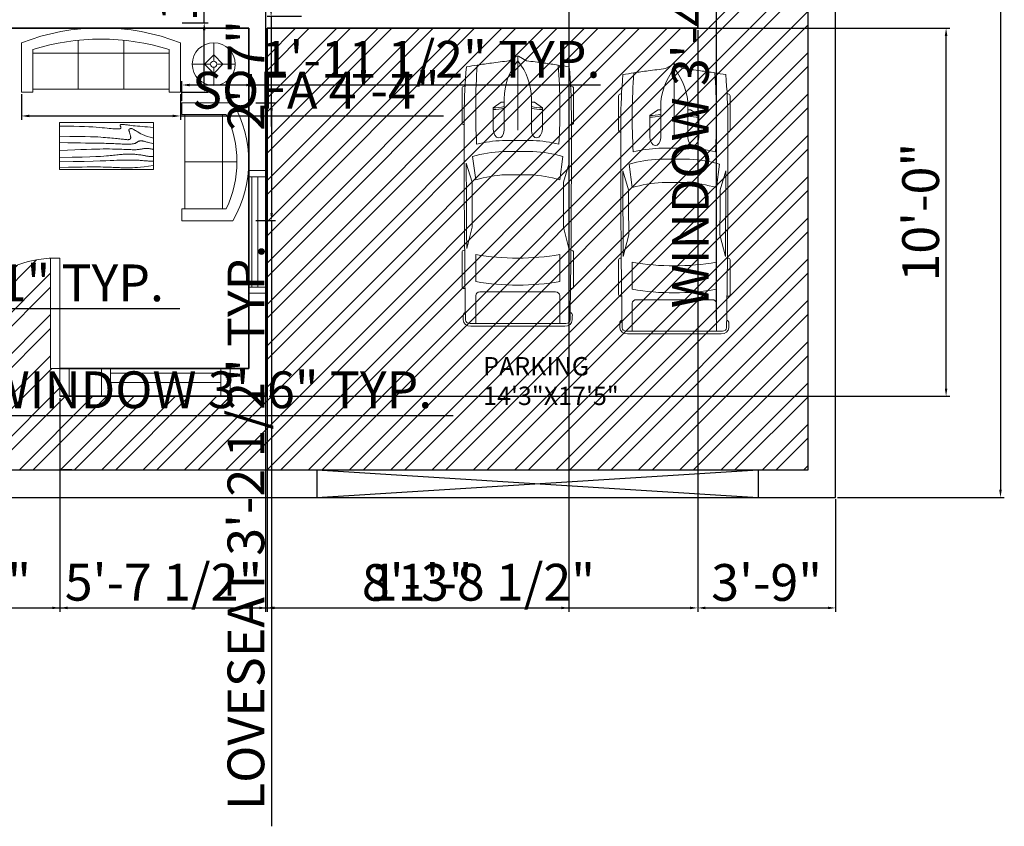
# Model space of a CAD drawing. Units: inches. Extents: x 2297 to 3143, y 440 to 1351.
# Tile 3 of 6: x 2725 to 3047, y 440 to 703. Entities that reach past the tile are written whole.
import ezdxf

# ---------------------------------------------------------------- set-up
doc = ezdxf.new("R2010")
doc.units = ezdxf.units.IN
for name, color, linetype, lineweight in [('A-ANNO-DIMS', 2, 'Continuous', 18), ('A-AREA-IDEN', 7, 'Continuous', 18), ('A-DOOR', 4, 'Continuous', 20), ('A-FURN', 8, 'Continuous', 18), ('A-GLAZ', 4, 'Continuous', 18), ('A-WALL', 7, 'Continuous', 35), ('C-PKNG-VEH', 8, 'Continuous', 13), ('C-PROP', 7, 'Continuous', 25), ('C-SITE-PATT', 252, 'Continuous', 13), ('E-LITE', 9, 'Continuous', 13)]:
    doc.layers.add(name, color=color, linetype=linetype, lineweight=lineweight)
doc.styles.get("Standard").update_dxf_attribs({"font": 'arial.ttf'})
doc.dimstyles.new('ISO-25', dxfattribs={"dimtxt": 12, "dimasz": 2.5, "dimexe": 1.25, "dimexo": 0.625, "dimtad": 1, "dimdec": 1, "dimlunit": 3, "dimtxsty": 'Standard', "dimcen": 2.5, "dimadec": 0, "dimazin": 0, "dimtfac": 1, "dimtdec": 1, "dimtmove": 0, "dimatfit": 3, "dimfxl": 1, "dimarcsym": 0})

# ---------------------------------------------------------------- blocks, each defined once
blk = doc.blocks.new('Sofa - Roundback Loveseat 5 ft.')
for p, q in [((0, -32.44198), (0, -5.99998)), ((-24, -33.99998), (-24, -11.46958)), ((-23.9998, -13.38178), (23.99986, -13.38178)), ((24.00004, -33.99998), (24.00004, -11.46958)), ((-24, -32.44198), (24.00004, -32.44198))]:
    blk.add_line(p, q)
for points in [[(-24, -33.99998), (-30, -33.99998), (-30, -7.99998)], [(30.00004, -7.99998), (30.00004, -33.99998), (24.00004, -33.99998)]]:
    blk.add_lwpolyline(points)
for centre, radius, start, end in [((0, -60.24998), 60.24998, 60.13715, 119.8628), ((0, -61.38438), 55.38444, 64.32083, 115.6792)]:
    blk.add_arc(centre, radius, start, end)
blk = doc.blocks.new('Table - Rectangular Woodgrain 60 x 30 in.')
for p, q in [((0, 0), (0, -30)), ((60, 0), (0, 0)), ((60, -30), (60, 0)), ((0, -30), (60, -30))]:
    blk.add_line(p, q)
for points in [[(0, -2.4), (4.8155, -2.418), (9.0302, -2.4688), (12.709, -2.5477), (15.9167, -2.65), (18.7181, -2.7711), (21.1781, -2.9063), (23.3616, -3.0508), (25.3333, -3.2), (27.1477, -3.3495), (28.8172, -3.4958), (30.3437, -3.636), (31.7291, -3.7667), (32.9756, -3.8849), (34.0849, -3.9875), (35.059, -4.0714), (35.9, -4.1334), (36.6114, -4.1711), (37.2041, -4.1854), (37.6906, -4.1779), (38.0833, -4.15), (38.3948, -4.1034), (38.6375, -4.0396), (38.8239, -3.9602), (38.9666, -3.8667), (39.0764, -3.7608), (39.1573, -3.6448), (39.2116, -3.521), (39.2416, -3.3917), (39.2498, -3.2593), (39.2385, -3.1261), (39.21, -2.9944), (39.1666, -2.8667), (39.111, -2.7447), (39.0468, -2.6281), (38.978, -2.5163), (38.9083, -2.4083), (38.8418, -2.3035), (38.7823, -2.201), (38.7337, -2.1001), (38.7, -2), (38.6844, -1.9003), (38.6875, -1.8021), (38.7094, -1.707), (38.75, -1.6167), (38.8094, -1.5326), (38.8875, -1.4563), (38.9844, -1.3893), (39.1, -1.3333), (39.2351, -1.2896), (39.3937, -1.2583), (39.5804, -1.2396), (39.8, -1.2333), (40.057, -1.2396), (40.3562, -1.2583), (40.7023, -1.2896), (41.1, -1.3333), (41.5547, -1.3895), (42.0755, -1.4573), (42.6721, -1.5361), (43.3542, -1.625), (44.1316, -1.7233), (45.014, -1.8302), (46.0114, -1.9449), (47.1333, -2.0667), (48.3862, -2.1947), (49.7625, -2.3281), (51.2513, -2.4663), (52.8416, -2.6083), (54.5226, -2.7535), (56.2833, -2.9011), (58.1127, -3.0501), (60, -3.2)], [(0, -9.2), (6.5759, -9.0858), (11.9385, -9.0365), (16.2527, -9.0418), (19.6833, -9.0917), (22.3952, -9.1759), (24.5531, -9.2844), (26.322, -9.4069), (27.8666, -9.5333), (29.3241, -9.6553), (30.7203, -9.7719), (32.0532, -9.8837), (33.3208, -9.9917), (34.5213, -10.0965), (35.6526, -10.199), (36.7128, -10.2999), (37.7, -10.4), (38.6129, -10.4996), (39.4531, -10.5969), (40.223, -10.6895), (40.925, -10.775), (41.5613, -10.8512), (42.1344, -10.9156), (42.6465, -10.966), (43.1, -11), (43.4976, -11.0158), (43.8437, -11.0136), (44.143, -10.9942), (44.4, -10.9583), (44.6195, -10.9069), (44.8062, -10.8406), (44.9648, -10.7603), (45.1, -10.6667), (45.2155, -10.5598), (45.3114, -10.4365), (45.3871, -10.2929), (45.4416, -10.125), (45.4743, -9.929), (45.4844, -9.7011), (45.4709, -9.4371), (45.4333, -9.1333), (45.3716, -8.7883), (45.2896, -8.4104), (45.1919, -8.0107), (45.0833, -7.6), (44.9685, -7.1893), (44.8521, -6.7896), (44.7388, -6.4117), (44.6333, -6.0667), (44.54, -5.7628), (44.4614, -5.4979), (44.4001, -5.2675), (44.3583, -5.0667), (44.3384, -4.8909), (44.3427, -4.7354), (44.3736, -4.5956), (44.4333, -4.4667), (44.5236, -4.3453), (44.6427, -4.2333), (44.7884, -4.1339), (44.9583, -4.05), (45.1501, -3.9849), (45.3614, -3.9417), (45.59, -3.9234), (45.8333, -3.9333), (46.0915, -3.9749), (46.3734, -4.0531), (46.6906, -4.1736), (47.0542, -4.3417), (47.4756, -4.5629), (47.9661, -4.8427), (48.5372, -5.1866), (49.2, -5.6), (49.9676, -6.0844), (50.8594, -6.625), (51.8965, -7.2031), (53.1, -7.8), (54.491, -8.3969), (56.0906, -8.975), (57.9199, -9.5156), (60, -10)], [(0, -12.8), (5.1847, -12.9322), (9.6213, -13.0323), (13.3963, -13.1059), (16.5958, -13.1583), (19.3063, -13.1952), (21.614, -13.2219), (23.6054, -13.2439), (25.3666, -13.2667), (26.9728, -13.2947), (28.4531, -13.3281), (29.8256, -13.3663), (31.1083, -13.4083), (32.3191, -13.4535), (33.476, -13.501), (34.597, -13.5501), (35.7, -13.6), (36.7984, -13.6497), (37.8875, -13.6979), (38.9578, -13.743), (40, -13.7833), (41.0047, -13.8174), (41.9625, -13.8438), (42.864, -13.8607), (43.7, -13.8667), (44.4631, -13.8604), (45.1552, -13.8417), (45.7801, -13.8104), (46.3416, -13.7667), (46.8439, -13.7104), (47.2906, -13.6417), (47.6858, -13.5604), (48.0333, -13.4667), (48.3375, -13.3608), (48.6042, -13.2448), (48.8396, -13.121), (49.05, -12.9917), (49.2417, -12.8593), (49.4208, -12.7261), (49.5937, -12.5944), (49.7667, -12.4667), (49.9452, -12.3451), (50.1323, -12.2313), (50.3303, -12.1268), (50.5416, -12.0333), (50.7686, -11.9524), (51.0135, -11.8854), (51.2788, -11.8341), (51.5666, -11.8), (51.8785, -11.7843), (52.2116, -11.7865), (52.562, -11.8059), (52.926, -11.8417), (53.2998, -11.8931), (53.6795, -11.9594), (54.0614, -12.0397), (54.4416, -12.1333), (54.8223, -12.2401), (55.2293, -12.3625), (55.6942, -12.5037), (56.2489, -12.6667), (56.9251, -12.8547), (57.7545, -13.0708), (58.7689, -13.3182), (60, -13.6)], [(0, -18), (5.124, -17.7273), (9.6609, -17.5057), (13.6705, -17.3303), (17.2125, -17.1958), (20.3467, -17.0973), (23.1328, -17.0297), (25.6307, -16.9878), (27.9, -16.9667), (29.9928, -16.9617), (31.9302, -16.9703), (33.7254, -16.9907), (35.3917, -17.0208), (36.9423, -17.0588), (38.3906, -17.1026), (39.7499, -17.1503), (41.0333, -17.2), (42.2519, -17.2496), (43.4073, -17.2969), (44.4986, -17.3395), (45.525, -17.375), (46.4858, -17.4012), (47.3802, -17.4156), (48.2074, -17.416), (48.9667, -17.4), (49.6583, -17.3662), (50.2872, -17.3167), (50.8595, -17.2547), (51.3812, -17.1833), (51.8584, -17.1057), (52.2971, -17.025), (52.7034, -16.9443), (53.0833, -16.8667), (53.443, -16.7951), (53.789, -16.7313), (54.128, -16.6768), (54.4666, -16.6334), (54.8115, -16.6024), (55.1693, -16.5854), (55.5465, -16.5841), (55.95, -16.6), (56.3828, -16.6337), (56.8346, -16.6823), (57.2915, -16.7418), (57.7396, -16.8084), (58.165, -16.878), (58.5539, -16.9469), (58.8924, -17.0111), (59.1666, -17.0667), (59.3679, -17.1107), (59.5078, -17.1438), (59.6032, -17.1675), (59.6708, -17.1833), (59.7275, -17.193), (59.7901, -17.1979), (59.8753, -17.1998), (60, -17.2)], [(0, -22.4), (8.0098, -22.2501), (14.4094, -22.1011), (19.4168, -21.9535), (23.25, -21.8083), (26.1269, -21.6663), (28.2656, -21.5281), (29.884, -21.3947), (31.2, -21.2667), (32.3967, -21.1448), (33.5172, -21.0292), (34.5697, -20.9198), (35.5625, -20.8167), (36.5037, -20.7198), (37.4015, -20.6292), (38.2642, -20.5448), (39.1, -20.4667), (39.9164, -20.3951), (40.7187, -20.3313), (41.5117, -20.2768), (42.3, -20.2333), (43.0883, -20.2024), (43.8812, -20.1854), (44.6836, -20.1841), (45.5, -20.2), (46.3328, -20.234), (47.1747, -20.2844), (48.0163, -20.3488), (48.8479, -20.425), (49.66, -20.5106), (50.4429, -20.6031), (51.1872, -20.7004), (51.8833, -20.8), (52.5246, -20.8999), (53.1166, -20.9995), (53.6681, -21.0983), (54.1875, -21.1958), (54.6834, -21.2919), (55.1646, -21.3859), (55.6394, -21.4777), (56.1167, -21.5667), (56.6028, -21.6515), (57.0961, -21.7266), (57.5929, -21.7852), (58.0896, -21.8208), (58.5823, -21.8268), (59.0674, -21.7964), (59.5412, -21.723), (60, -21.6)], [(0, -25.2), (8.6355, -25.0504), (15.7026, -24.9031), (21.4049, -24.7606), (25.9458, -24.625), (29.529, -24.4988), (32.3578, -24.3844), (34.6359, -24.284), (36.5667, -24.2), (38.3213, -24.1341), (39.9417, -24.0854), (41.437, -24.0523), (42.8167, -24.0333), (44.0901, -24.0268), (45.2667, -24.0313), (46.3557, -24.0451), (47.3667, -24.0667), (48.309, -24.0947), (49.1928, -24.1287), (50.0284, -24.168), (50.826, -24.2125), (51.5959, -24.2617), (52.3483, -24.3151), (53.0935, -24.3725), (53.8417, -24.4334), (54.6009, -24.497), (55.3699, -24.561), (56.1454, -24.6226), (56.9239, -24.6792), (57.7021, -24.7279), (58.4764, -24.7662), (59.2435, -24.7911), (60, -24.8)], [(0, -28.8), (5.6867, -28.6681), (10.45, -28.5698), (14.407, -28.5012), (17.675, -28.4584), (20.3711, -28.4374), (22.6125, -28.4344), (24.5164, -28.4455), (26.2, -28.4667), (27.762, -28.4947), (29.2276, -28.5281), (30.6033, -28.5663), (31.8958, -28.6084), (33.1118, -28.6535), (34.2578, -28.7011), (35.3405, -28.7501), (36.3666, -28.8), (37.3443, -28.8497), (38.288, -28.8974), (39.2137, -28.9412), (40.1375, -28.9792), (41.0753, -29.0093), (42.0432, -29.0297), (43.0572, -29.0384), (44.1333, -29.0333), (45.2936, -29.0114), (46.5843, -28.9641), (48.0579, -28.8816), (49.7666, -28.7542), (51.7629, -28.5721), (54.0989, -28.3255), (56.8272, -28.0048), (60, -27.6)]]:
    blk.add_lwpolyline(points)
blk = doc.blocks.new('Sofa - Roundback 7 ft.')
for p, q in [((-12.00002, -32.4421), (-12.00003, -6.5971)), ((11.99997, -32.4421), (11.99998, -6.5971)), ((-36.000027, -34), (-36.000027, -11.4696)), ((-35.999844, -13.3819), (35.9998, -13.3819)), ((35.99998, -34), (35.99998, -11.4696)), ((-36.000027, -32.4421), (35.99998, -32.4421))]:
    blk.add_line(p, q)
for points in [[(-36.000027, -34), (-42.000027, -34), (-42.000027, -8)], [(41.99998, -8), (41.99998, -34), (35.99998, -34)]]:
    blk.add_lwpolyline(points)
for centre, radius, start, end in [((0, -114.25), 114.25, 68.43141, 111.5686), ((-0.00001, -127.1968), 121.1968, 72.72033, 107.2797)]:
    blk.add_arc(centre, radius, start, end)
blk = doc.blocks.new('*U14')
for p, q in [((21.1, 37.41), (21.1, 36.83)), ((46.55, 38.89), (22.35, 38.89)), ((47.8, 37.39), (47.8, 37.41)), ((87.99, 31.87), (74.76, 35.92)), ((134.31, 35.6), (119.29, 31.78)), ((135.45, 37.07), (135.45, 37.41)), ((136.7, 38.89), (160.9, 38.89)), ((162.15, 37.41), (162.15, 36.77)), ((70.03, 31.54), (86.41, 29.35)), ((138.42, 29.35), (157.25, 29.35)), ((186.47, 29.35), (167.01, 29.35)), ((186.47, -33.5), (186.47, 33.5)), ((188.4, -32.76), (188.4, 32.76)), ((164.52, 26.39), (164.52, -26.39)), ((32.27, 11.63), (36.13, 17.17)), ((36.13, 17.17), (50.94, 17.17)), ((29.77, 9.51), (51.68, 9.51)), ((32.12, 9.51), (32.12, 11.15)), ((58.92, -10.77), (58.92, 10.77)), ((66.55, -10.53), (66.55, 10.53)), ((82.74, 8.5), (82.74, -8.5)), ((186.47, -10.53), (186.47, 10.53)), ((3.27, 6.13), (0.1, 0.41)), ((0, 0), (51.68, 0)), ((0.1, -0.41), (3.27, -6.13)), ((29.77, -9.51), (51.68, -9.51)), ((32.12, -9.51), (32.12, -11.15)), ((32.27, -11.63), (36.13, -17.17)), ((36.13, -17.17), (50.94, -17.17)), ((86.41, -29.35), (70.03, -31.54)), ((87.99, -31.87), (74.76, -35.92)), ((134.31, -35.6), (119.29, -31.78)), ((157.25, -29.35), (138.42, -29.35)), ((167.01, -29.35), (186.47, -29.35)), ((21.1, -37.41), (21.1, -36.83)), ((46.55, -38.89), (22.35, -38.89)), ((47.8, -37.39), (47.8, -37.41)), ((135.45, -37.07), (135.45, -37.41)), ((136.7, -38.89), (160.9, -38.89)), ((162.15, -37.41), (162.15, -36.77))]:
    blk.add_line(p, q)
for centre, major_axis, ratio, start_param, end_param in [((266.03, -27.52), (0, 313.31), 0.842304, 1.367076, 1.39176), ((41.19, -490.86), (0, 528.23), 0.842304, 0.00281, 0.075598), ((22.35, 37.41), (0, -1.48), 0.842304, 3.141593, 4.712389), ((64.48, -10555.62), (0, 10593.03), 0.842304, -0.013397, 0.002797), ((46.55, 37.41), (0, 1.48), 0.842304, -1.570796, 0), ((64.48, -10555.62), (0, -10591.55), 0.842304, 3.133765, 3.140441), ((136.7, 37.41), (0, -1.48), 0.842304, 3.141593, 4.712389), ((160.9, 37.41), (0, 1.48), 0.842304, -1.570796, 0), ((180.63, 35.84), (0, 2.22), 0.842304, -0.013017, 1.249894), ((64.48, -10556.36), (0, 10595.31), 0.842304, -0.013397, -0.013017), ((183.98, 33.5), (0, -2.96), 0.842304, 1.570796, 3.128196), ((183.98, 32.76), (0, -5.25), 0.842304, 1.570796, 3.128196), ((259.18, -27.52), (0, -305.3), 0.842304, 4.528606, 4.561838), ((37.47, -593.96), (0, -623.33), 0.842304, 3.096046, 3.200911), ((134.4, 5.39), (0, -89.78), 0.842304, 4.449482, 4.652344), ((135.29, 5.39), (0, 81.77), 0.842304, 1.245306, 1.50788), ((149.6, 2.8), (0, -79.58), 0.842304, 4.372215, 4.640744), ((95.79, -3666.35), (0, -3698.24), 0.842304, 3.134049, 3.144098), ((17.08, 0), (0, 147.02), 0.842304, 4.511394, 4.913384), ((35.91, 0), (0, 147.02), 0.842304, 4.511394, 4.913384), ((167.01, 26.39), (0, 2.96), 0.842304, 0, 1.570796), ((-204.49, 52.4), (0, -250.96), 0.842304, 1.385369, 1.434372), ((13.04, 17.01), (0, 27.42), 0.842304, 4.435146, 4.718221), ((14.2, 17.01), (0, 27.42), 0.842304, 4.435146, 4.718221), ((50.79, 13.34), (6.34, -0.36), 0.603834, -1.395552, 1.581315), ((29.77, -46.66), (0, 56.17), 0.842304, 0, 0.590319), ((32.75, 11.15), (0, 0.74), 0.842304, 0.879714, 1.570796), ((0.62, 0), (0, -0.74), 0.842304, 4.131459, 5.293319), ((-204.49, -52.4), (0, 250.96), 0.842304, -1.434372, -1.385369), ((29.77, 46.66), (0, 56.17), 0.842304, 2.551274, 3.141593), ((32.75, -11.15), (0, -0.74), 0.842304, 4.712389, 5.403472), ((13.04, -17.01), (0, -27.42), 0.842304, 1.564964, 1.848039), ((14.2, -17.01), (0, -27.42), 0.842304, 1.564964, 1.848039), ((134.4, -5.39), (0, -89.78), 0.842304, -1.510751, -1.307889), ((135.29, -5.39), (0, -81.77), 0.842304, -1.50788, -1.245306), ((149.6, -2.8), (0, -79.58), 0.842304, -1.499151, -1.230623), ((259.18, 27.52), (0, 305.3), 0.842304, 1.721348, 1.754579), ((167.01, -26.39), (0, -2.96), 0.842304, 4.712389, 6.283185), ((266.03, 27.52), (0, 313.31), 0.842304, 1.749832, 1.774517), ((37.47, 593.96), (0, -623.33), 0.842304, -0.059319, 0.045547), ((95.79, 3666.35), (0, -3698.24), 0.842304, -0.002505, 0.007544), ((183.98, -33.5), (0, 2.96), 0.842304, 3.15499, 4.712389), ((183.98, -32.76), (0, -5.25), 0.842304, 0.013397, 1.570796), ((41.19, 490.86), (0, -528.23), 0.842304, -0.075598, -0.00281), ((22.35, -37.41), (0, 1.48), 0.842304, 1.570796, 3.141593), ((64.48, 10555.62), (0, 10593.03), 0.842304, 3.138796, 3.15499), ((46.55, -37.41), (0, -1.48), 0.842304, 0, 1.570796), ((64.48, 10555.62), (0, -10591.55), 0.842304, 0.001152, 0.007828), ((136.7, -37.41), (0, -1.48), 0.842304, -1.570796, 0), ((160.9, -37.41), (0, 1.48), 0.842304, 3.141593, 4.712389), ((180.63, -35.84), (0, -2.22), 0.842304, -1.249894, 0.013017), ((64.48, 10556.36), (0, 10595.31), 0.842304, 3.15461, 3.15499)]:
    blk.add_ellipse(centre, major_axis=major_axis, ratio=ratio, start_param=start_param, end_param=end_param)
at = {"extrusion": (0, 0, -1)}
blk.add_ellipse((50.79, -13.34), major_axis=(6.34, 0.36), ratio=0.603834, start_param=-1.395552, end_param=1.581315, dxfattribs=at)
blk = doc.blocks.new('*D18')
at = {"layer": 'A-ANNO-DIMS', "color": 0, "lineweight": -2, "transparency": 16777216}
for p, q in [((2993.8, 1207.63), (3046.74, 1207.63)), ((3045.49, 1205.13), (3045.49, 550.13)), ((2992.32, 547.63), (3046.74, 547.63))]:
    blk.add_line(p, q, dxfattribs=at)
at = {"layer": 'A-ANNO-DIMS', "color": 0, "transparency": 16777216}
for points in [[(3045.07, 1205.13), (3045.91, 1205.13), (3045.49, 1207.63)], [(3045.07, 550.13), (3045.91, 550.13), (3045.49, 547.63)]]:
    blk.add_solid(points, dxfattribs=at)
at = {"layer": 'Defpoints', "color": 0, "transparency": 16777216}
for p in [(2993.18, 1207.63), (2991.69, 547.63), (3045.49, 547.63)]:
    blk.add_point(p, dxfattribs=at)
at = {"layer": 'A-ANNO-DIMS', "color": 0, "transparency": 16777216, "insert": (3038.76, 877.63), "char_height": 12, "attachment_point": 5, "rotation": 90}
blk.add_mtext("55'", dxfattribs=at)
blk = doc.blocks.new('Lamp - Table')
for p, q in [((0, 7), (0, 1)), ((-1, 0), (-7, 0)), ((0, 3), (-3, 0)), ((-3, 0), (0, -3)), ((3, 0), (0, 3)), ((0, -3), (3, 0)), ((1, 0), (7, 0)), ((0, -1), (0, -7))]:
    blk.add_line(p, q)
for radius in [7, 1]:
    blk.add_circle((0, 0), radius)
blk = doc.blocks.new('WIN-36IN-6IN-WALL')
for p, q in [((6, 40), (0, 40)), ((6, 38), (0, 38)), ((3, 38), (3, 2)), ((5, 38), (5, 2)), ((0, 2), (6, 2)), ((0, 0), (6, 0))]:
    blk.add_line(p, q)
blk = doc.blocks.new('WIN-36IN-9IN-WALL')
for p, q in [((0, 9), (0, 0)), ((3, 9), (3, 0)), ((3, 7.5), (39, 7.5)), ((39, 0), (39, 9)), ((42, 0), (42, 9)), ((3, 4.5), (39, 4.5))]:
    blk.add_line(p, q)
blk = doc.blocks.new('*D31')
at = {"layer": 'A-ANNO-DIMS', "color": 0, "lineweight": -2, "transparency": 16777216}
for p, q in [((2947.32, 801.2), (2953.94, 801.2)), ((2952.69, 798.7), (2952.69, 763.7)), ((2947.32, 761.2), (2953.94, 761.2)), ((2952.69, 761.2), (2952.69, 605.6))]:
    blk.add_line(p, q, dxfattribs=at)
at = {"layer": 'A-ANNO-DIMS', "color": 0, "transparency": 16777216}
for points in [[(2952.28, 798.7), (2953.11, 798.7), (2952.69, 801.2)], [(2952.28, 763.7), (2953.11, 763.7), (2952.69, 761.2)]]:
    blk.add_solid(points, dxfattribs=at)
at = {"layer": 'Defpoints', "color": 0, "transparency": 16777216}
for p in [(2946.69, 801.2), (2946.69, 761.2), (2952.69, 761.2)]:
    blk.add_point(p, dxfattribs=at)
at = {"layer": 'A-ANNO-DIMS', "color": 0, "transparency": 16777216, "insert": (2945.85, 682.15), "char_height": 12, "attachment_point": 5, "rotation": 90}
blk.add_mtext('WINDOW 3\'-4" TYP.', dxfattribs=at)
blk = doc.blocks.new('*D35')
at = {"layer": 'A-ANNO-DIMS', "color": 0, "lineweight": -2, "transparency": 16777216}
for p, q in [((2568, 612.02), (2568, 607.95)), ((2591, 612.02), (2591, 607.95)), ((2570.5, 609.2), (2588.5, 609.2)), ((2591, 609.2), (2777.67, 609.2))]:
    blk.add_line(p, q, dxfattribs=at)
at = {"layer": 'A-ANNO-DIMS', "color": 0, "transparency": 16777216}
for points in [[(2570.5, 609.61), (2570.5, 608.78), (2568, 609.2)], [(2588.5, 609.61), (2588.5, 608.78), (2591, 609.2)]]:
    blk.add_solid(points, dxfattribs=at)
at = {"layer": 'Defpoints', "color": 0, "transparency": 16777216}
for p in [(2568, 612.65), (2591, 612.65), (2591, 609.2)]:
    blk.add_point(p, dxfattribs=at)
at = {"layer": 'A-ANNO-DIMS', "color": 0, "transparency": 16777216, "insert": (2685.59, 616.03), "char_height": 12, "attachment_point": 5}
blk.add_mtext('COMPUTER 1\'-11" TYP.', dxfattribs=at)
blk = doc.blocks.new('*D47')
at = {"layer": 'A-ANNO-DIMS', "color": 0, "lineweight": -2, "transparency": 16777216}
for p, q in [((2802.53, 676.34), (2808.92, 676.34)), ((2807.67, 673.84), (2807.67, 640.37)), ((2802.53, 637.87), (2808.92, 637.87)), ((2807.67, 637.87), (2807.67, 440.38))]:
    blk.add_line(p, q, dxfattribs=at)
at = {"layer": 'A-ANNO-DIMS', "color": 0, "transparency": 16777216}
for points in [[(2807.26, 673.84), (2808.09, 673.84), (2807.67, 676.34)], [(2807.26, 640.37), (2808.09, 640.37), (2807.67, 637.87)]]:
    blk.add_solid(points, dxfattribs=at)
at = {"layer": 'Defpoints', "color": 0, "transparency": 16777216}
for p in [(2801.9, 676.34), (2801.9, 637.87), (2807.67, 637.87)]:
    blk.add_point(p, dxfattribs=at)
at = {"layer": 'A-ANNO-DIMS', "color": 0, "transparency": 16777216, "insert": (2800.83, 537.87), "char_height": 12, "attachment_point": 5, "rotation": 90}
blk.add_mtext('LOVESEAT 3\'-2 1/2" TYP.', dxfattribs=at)
blk = doc.blocks.new('*D48')
at = {"layer": 'A-ANNO-DIMS', "color": 0, "lineweight": -2, "transparency": 16777216}
for p, q in [((2778.39, 676.96), (2778.39, 683.36)), ((2780.89, 682.11), (2799.4, 682.11)), ((2801.9, 676.96), (2801.9, 683.36)), ((2801.9, 682.11), (2914.95, 682.11))]:
    blk.add_line(p, q, dxfattribs=at)
at = {"layer": 'A-ANNO-DIMS', "color": 0, "transparency": 16777216}
for points in [[(2780.89, 682.52), (2780.89, 681.69), (2778.39, 682.11)], [(2799.4, 682.52), (2799.4, 681.69), (2801.9, 682.11)]]:
    blk.add_solid(points, dxfattribs=at)
at = {"layer": 'Defpoints', "color": 0, "transparency": 16777216}
for p in [(2801.9, 682.11), (2778.39, 676.34), (2801.9, 676.34)]:
    blk.add_point(p, dxfattribs=at)
at = {"layer": 'A-ANNO-DIMS', "color": 0, "transparency": 16777216, "insert": (2859.68, 688.94), "char_height": 12, "attachment_point": 5}
blk.add_mtext('1\'-11 1/2" TYP.', dxfattribs=at)
blk = doc.blocks.new('*D50')
at = {"layer": 'A-ANNO-DIMS', "color": 0, "lineweight": -2, "transparency": 16777216}
for p, q in [((2817.45, 735.15), (2806.26, 735.15)), ((2807.51, 732.65), (2807.51, 706.9)), ((2817.45, 704.4), (2806.26, 704.4)), ((2807.51, 704.4), (2807.51, 668.54))]:
    blk.add_line(p, q, dxfattribs=at)
at = {"layer": 'A-ANNO-DIMS', "color": 0, "transparency": 16777216}
for points in [[(2807.09, 732.65), (2807.92, 732.65), (2807.51, 735.15)], [(2807.09, 706.9), (2807.92, 706.9), (2807.51, 704.4)]]:
    blk.add_solid(points, dxfattribs=at)
at = {"layer": 'Defpoints', "color": 0, "transparency": 16777216}
for p in [(2818.08, 735.15), (2807.51, 704.4), (2818.08, 704.4)]:
    blk.add_point(p, dxfattribs=at)
at = {"layer": 'A-ANNO-DIMS', "color": 0, "transparency": 16777216, "insert": (2800.86, 685.22), "char_height": 12, "attachment_point": 5, "rotation": 90}
blk.add_mtext('2\'-7"', dxfattribs=at)
blk = doc.blocks.new('*D51')
at = {"layer": 'A-ANNO-DIMS', "color": 0, "lineweight": -2, "transparency": 16777216}
for p, q in [((2726.08, 679.16), (2726.08, 670.76)), ((2777.91, 679.16), (2777.91, 670.76)), ((2728.58, 672.01), (2775.41, 672.01)), ((2777.91, 672.01), (2863.8, 672.01))]:
    blk.add_line(p, q, dxfattribs=at)
at = {"layer": 'A-ANNO-DIMS', "color": 0, "transparency": 16777216}
for points in [[(2728.58, 672.43), (2728.58, 671.6), (2726.08, 672.01)], [(2775.41, 672.43), (2775.41, 671.6), (2777.91, 672.01)]]:
    blk.add_solid(points, dxfattribs=at)
at = {"layer": 'Defpoints', "color": 0, "transparency": 16777216}
for p in [(2726.08, 679.79), (2777.91, 679.79), (2777.91, 672.01)]:
    blk.add_point(p, dxfattribs=at)
at = {"layer": 'A-ANNO-DIMS', "color": 0, "transparency": 16777216, "insert": (2822.1, 678.85), "char_height": 12, "attachment_point": 5}
blk.add_mtext('SOFA 4\'-4"', dxfattribs=at)
blk = doc.blocks.new('*D52')
at = {"layer": 'A-ANNO-DIMS', "color": 0, "lineweight": -2, "transparency": 16777216}
for p, q in [((2785.68, 702.41), (2785.68, 774.21)), ((2778.53, 702.41), (2786.93, 702.41)), ((2785.68, 682.29), (2785.68, 699.91)), ((2778.53, 679.79), (2786.93, 679.79))]:
    blk.add_line(p, q, dxfattribs=at)
at = {"layer": 'A-ANNO-DIMS', "color": 0, "transparency": 16777216}
for points in [[(2785.26, 699.91), (2786.09, 699.91), (2785.68, 702.41)], [(2785.26, 682.29), (2786.09, 682.29), (2785.68, 679.79)]]:
    blk.add_solid(points, dxfattribs=at)
at = {"layer": 'Defpoints', "color": 0, "transparency": 16777216}
for p in [(2777.91, 702.41), (2785.68, 702.41), (2777.91, 679.79)]:
    blk.add_point(p, dxfattribs=at)
at = {"layer": 'A-ANNO-DIMS', "color": 0, "transparency": 16777216, "insert": (2778.85, 739.56), "char_height": 12, "attachment_point": 5, "rotation": 90}
blk.add_mtext('1\'-10 1/2"', dxfattribs=at)
blk = doc.blocks.new('*D59')
at = {"layer": 'A-ANNO-DIMS', "color": 0, "lineweight": -2, "transparency": 16777216}
for p, q in [((2608.99, 580.01), (2608.99, 573.08)), ((2650.99, 580.01), (2650.99, 573.08)), ((2611.49, 574.33), (2648.49, 574.33)), ((2650.99, 574.33), (2866.94, 574.33))]:
    blk.add_line(p, q, dxfattribs=at)
at = {"layer": 'A-ANNO-DIMS', "color": 0, "transparency": 16777216}
for points in [[(2611.49, 574.75), (2611.49, 573.92), (2608.99, 574.33)], [(2648.49, 574.75), (2648.49, 573.92), (2650.99, 574.33)]]:
    blk.add_solid(points, dxfattribs=at)
at = {"layer": 'Defpoints', "color": 0, "transparency": 16777216}
for p in [(2608.99, 580.63), (2650.99, 580.63), (2650.99, 574.33)]:
    blk.add_point(p, dxfattribs=at)
at = {"layer": 'A-ANNO-DIMS', "color": 0, "transparency": 16777216, "insert": (2760.21, 581.17), "char_height": 12, "attachment_point": 5}
blk.add_mtext('ENTRY WINDOW 3\'-6" TYP.', dxfattribs=at)
blk = doc.blocks.new('*D69')
at = {"layer": 'A-ANNO-DIMS', "color": 0, "lineweight": -2, "transparency": 16777216}
for p, q in [((2946.69, 700.01), (2946.69, 510.33)), ((2438.19, 580.01), (2438.19, 510.33)), ((2440.69, 511.58), (2944.19, 511.58))]:
    blk.add_line(p, q, dxfattribs=at)
at = {"layer": 'A-ANNO-DIMS', "color": 0, "transparency": 16777216}
for points in [[(2440.69, 512), (2440.69, 511.17), (2438.19, 511.58)], [(2944.19, 512), (2944.19, 511.17), (2946.69, 511.58)]]:
    blk.add_solid(points, dxfattribs=at)
at = {"layer": 'Defpoints', "color": 0, "transparency": 16777216}
for p in [(2946.69, 700.63), (2438.19, 580.63), (2946.69, 511.58)]:
    blk.add_point(p, dxfattribs=at)
at = {"layer": 'A-ANNO-DIMS', "color": 0, "transparency": 16777216, "insert": (2692.44, 518.41), "char_height": 12, "attachment_point": 5}
blk.add_mtext('42\'-4 1/2"', dxfattribs=at)
blk = doc.blocks.new('*D72')
at = {"layer": 'A-ANNO-DIMS', "color": 0, "lineweight": -2, "transparency": 16777216}
for p, q in [((2946.69, 700.01), (2946.69, 510.33)), ((2991.69, 547.01), (2991.69, 510.33)), ((2949.19, 511.58), (2989.19, 511.58))]:
    blk.add_line(p, q, dxfattribs=at)
at = {"layer": 'A-ANNO-DIMS', "color": 0, "transparency": 16777216}
for points in [[(2949.19, 512), (2949.19, 511.17), (2946.69, 511.58)], [(2989.19, 512), (2989.19, 511.17), (2991.69, 511.58)]]:
    blk.add_solid(points, dxfattribs=at)
at = {"layer": 'Defpoints', "color": 0, "transparency": 16777216}
for p in [(2946.69, 700.63), (2991.69, 547.63), (2991.69, 511.58)]:
    blk.add_point(p, dxfattribs=at)
at = {"layer": 'A-ANNO-DIMS', "color": 0, "transparency": 16777216, "insert": (2969.19, 518.34), "char_height": 12, "attachment_point": 5}
blk.add_mtext('3\'-9"', dxfattribs=at)
blk = doc.blocks.new('*D74')
at = {"layer": 'A-ANNO-DIMS', "color": 0, "lineweight": -2, "transparency": 16777216}
for p, q in [((2806.82, 700.63), (3028.99, 700.63)), ((3027.74, 583.13), (3027.74, 698.13)), ((2806.82, 580.63), (3028.99, 580.63))]:
    blk.add_line(p, q, dxfattribs=at)
at = {"layer": 'A-ANNO-DIMS', "color": 0, "transparency": 16777216}
for points in [[(3027.33, 698.13), (3028.16, 698.13), (3027.74, 700.63)], [(3027.33, 583.13), (3028.16, 583.13), (3027.74, 580.63)]]:
    blk.add_solid(points, dxfattribs=at)
at = {"layer": 'Defpoints', "color": 0, "transparency": 16777216}
for p in [(2806.19, 700.63), (3027.74, 700.63), (2806.19, 580.63)]:
    blk.add_point(p, dxfattribs=at)
at = {"layer": 'A-ANNO-DIMS', "color": 0, "transparency": 16777216, "insert": (3020.99, 640.63), "char_height": 12, "attachment_point": 5, "rotation": 90}
blk.add_mtext('10\'-0"', dxfattribs=at)
blk = doc.blocks.new('*D75')
at = {"layer": 'A-ANNO-DIMS', "color": 0, "lineweight": -2, "transparency": 16777216}
for p, q in [((2806.19, 700.01), (2806.19, 510.33)), ((2946.69, 700.01), (2946.69, 510.33)), ((2808.69, 511.58), (2944.19, 511.58))]:
    blk.add_line(p, q, dxfattribs=at)
at = {"layer": 'A-ANNO-DIMS', "color": 0, "transparency": 16777216}
for points in [[(2808.69, 512), (2808.69, 511.17), (2806.19, 511.58)], [(2944.19, 512), (2944.19, 511.17), (2946.69, 511.58)]]:
    blk.add_solid(points, dxfattribs=at)
at = {"layer": 'Defpoints', "color": 0, "transparency": 16777216}
for p in [(2806.19, 700.63), (2946.69, 700.63), (2946.69, 511.58)]:
    blk.add_point(p, dxfattribs=at)
at = {"layer": 'A-ANNO-DIMS', "color": 0, "transparency": 16777216, "insert": (2876.44, 518.41), "char_height": 12, "attachment_point": 5}
blk.add_mtext('11\'-8 1/2"', dxfattribs=at)
blk = doc.blocks.new('*D79')
at = {"layer": 'A-ANNO-DIMS', "color": 0, "lineweight": -2, "transparency": 16777216}
for p, q in [((2805.69, 866.51), (2805.69, 510.33)), ((2904.69, 866.51), (2904.69, 510.33)), ((2808.19, 511.58), (2902.19, 511.58))]:
    blk.add_line(p, q, dxfattribs=at)
at = {"layer": 'A-ANNO-DIMS', "color": 0, "transparency": 16777216}
for points in [[(2808.19, 512), (2808.19, 511.17), (2805.69, 511.58)], [(2902.19, 512), (2902.19, 511.17), (2904.69, 511.58)]]:
    blk.add_solid(points, dxfattribs=at)
at = {"layer": 'Defpoints', "color": 0, "transparency": 16777216}
for p in [(2805.69, 867.13), (2904.69, 867.13), (2904.69, 511.58)]:
    blk.add_point(p, dxfattribs=at)
at = {"layer": 'A-ANNO-DIMS', "color": 0, "transparency": 16777216, "insert": (2855.19, 518.34), "char_height": 12, "attachment_point": 5}
blk.add_mtext('8\'-3"', dxfattribs=at)
blk = doc.blocks.new('*D81')
at = {"layer": 'A-ANNO-DIMS', "color": 0, "lineweight": -2, "transparency": 16777216}
for p, q in [((2666.57, 580.01), (2666.57, 510.33)), ((2738.57, 580.01), (2738.57, 510.33)), ((2669.07, 511.58), (2736.07, 511.58))]:
    blk.add_line(p, q, dxfattribs=at)
at = {"layer": 'A-ANNO-DIMS', "color": 0, "transparency": 16777216}
for points in [[(2669.07, 512), (2669.07, 511.17), (2666.57, 511.58)], [(2736.07, 512), (2736.07, 511.17), (2738.57, 511.58)]]:
    blk.add_solid(points, dxfattribs=at)
at = {"layer": 'Defpoints', "color": 0, "transparency": 16777216}
for p in [(2666.57, 580.63), (2738.57, 580.63), (2738.57, 511.58)]:
    blk.add_point(p, dxfattribs=at)
at = {"layer": 'A-ANNO-DIMS', "color": 0, "transparency": 16777216, "insert": (2702.57, 518.34), "char_height": 12, "attachment_point": 5}
blk.add_mtext('6\'-0"', dxfattribs=at)
blk = doc.blocks.new('*D82')
at = {"layer": 'A-ANNO-DIMS', "color": 0, "lineweight": -2, "transparency": 16777216}
for p, q in [((2738.57, 580.01), (2738.57, 510.33)), ((2806.19, 580.01), (2806.19, 510.33)), ((2741.07, 511.58), (2803.69, 511.58))]:
    blk.add_line(p, q, dxfattribs=at)
at = {"layer": 'A-ANNO-DIMS', "color": 0, "transparency": 16777216}
for points in [[(2741.07, 512), (2741.07, 511.17), (2738.57, 511.58)], [(2803.69, 512), (2803.69, 511.17), (2806.19, 511.58)]]:
    blk.add_solid(points, dxfattribs=at)
at = {"layer": 'Defpoints', "color": 0, "transparency": 16777216}
for p in [(2738.57, 580.63), (2806.19, 580.63), (2806.19, 511.58)]:
    blk.add_point(p, dxfattribs=at)
at = {"layer": 'A-ANNO-DIMS', "color": 0, "transparency": 16777216, "insert": (2772.38, 518.41), "char_height": 12, "attachment_point": 5}
blk.add_mtext('5\'-7 1/2"', dxfattribs=at)

msp = doc.modelspace()

# ---------------------------------------------------------------- hatches: boundary and pattern name
at = {"layer": 'C-SITE-PATT'}
h = msp.add_hatch(dxfattribs=at)
h.set_pattern_fill('ANSI32', color=256)
h.paths.add_polyline_path([(2438.19, 1198.63), (2402.19, 1198.63), (2402.19, 556.63), (2667.43, 556.63), (2742.43, 556.63), (2946.69, 556.63), (2982.69, 556.63), (2982.69, 1117.63), (2982.69, 1123.63), (2982.69, 1198.63), (2946.69, 1198.63), (2946.69, 1117.63), (2946.69, 700.63), (2806.19, 700.63), (2806.19, 580.63), (2738.57, 580.63), (2738.57, 589.63), (2735.57, 589.63), (2735.57, 625.63, 0.402069), (2702.6, 591.13, 0.401544), (2669.57, 625.63), (2669.57, 589.63), (2666.57, 589.63), (2666.57, 580.63), (2438.19, 580.63)])
h.paths.add_polyline_path([(2706.46, 558.2, -0.000472), (2706.46, 558.13, -0.000473)], flags=16)
h.paths.add_polyline_path([(2875.15, 576.11), (2920.92, 576.11), (2920.92, 585.31), (2875.15, 585.31)], flags=24)
h.paths.add_polyline_path([(2875.13, 585.74), (2915.96, 585.74), (2915.96, 595.05), (2875.13, 595.05)], flags=24)
h.paths.add_polyline_path([(2646.52, 1069.72), (2687.63, 1069.72), (2687.63, 1078.92), (2646.52, 1078.92)], flags=25)
h.paths.add_polyline_path([(2646.5, 1079.35), (2686.39, 1079.35), (2686.39, 1088.65), (2646.5, 1088.65)], flags=25)

# ---------------------------------------------------------------- linework, layer by layer
at = {"layer": 'A-DOOR'}
for p, q in [((2738.57, 589.63), (2738.57, 580.63)), ((2741.57, 589.63), (2741.57, 580.63))]:
    msp.add_line(p, q, dxfattribs=at)
msp.add_lwpolyline([(2738.57, 589.63), (2735.57, 589.63), (2735.57, 625.63), (2738.57, 625.63)], close=True, dxfattribs=at)
msp.add_arc((2737.07, 591.2), 34.47, 87.5057, 180.1084, dxfattribs=at)
at = {"layer": 'A-WALL'}
for p, q in [((2946.69, 700.63), (2946.69, 1117.63)), ((2642.19, 700.63), (2800.19, 700.63)), ((2800.19, 589.63), (2800.19, 700.63)), ((2806.19, 580.63), (2806.19, 700.63)), ((2806.19, 700.63), (2946.69, 700.63)), ((2738.57, 589.63), (2800.19, 589.63)), ((2738.57, 580.63), (2806.19, 580.63))]:
    msp.add_line(p, q, dxfattribs=at)
at = {"layer": 'C-PROP'}
for p, q in [((2982.69, 556.63), (2982.69, 1117.63)), ((2600.19, 556.63), (2742.43, 556.63)), ((2742.43, 556.63), (2946.69, 556.63)), ((2822.45, 556.63), (2822.45, 547.63)), ((2822.45, 556.63), (2966.45, 547.63)), ((2822.45, 547.63), (2966.45, 556.63)), ((2946.69, 556.63), (2982.69, 556.63)), ((2966.45, 556.63), (2966.45, 547.63))]:
    msp.add_line(p, q, dxfattribs=at)
for points in [[(2742.43, 547.63), (2991.69, 547.63), (2991.69, 1207.63), (2393.19, 1207.63)], [(2742.43, 556.63), (2739.43, 556.63)], [(2393.19, 547.63), (2742.43, 547.63)]]:
    msp.add_lwpolyline(points, dxfattribs=at)

# ---------------------------------------------------------------- block references
at = {"layer": 'A-FURN'}
for name, p, xscale, yscale, zscale in [('Sofa - Roundback 7 ft.', (2751.99, 700.76), 0.6169130188548803, 0.6169130188548803, 0.6169130188548803), ('Table - Rectangular Woodgrain 60 x 30 in.', (2738.49, 669.9), 0.5102167871031984, 0.5102167871031984, 0.5102167871031984)]:
    msp.add_blockref(name, p, dxfattribs=dict(at, xscale=xscale, yscale=yscale, zscale=zscale))
at = {"layer": 'A-FURN', "xscale": 0.6411223808005011, "yscale": 0.6411223808005011, "zscale": 0.6411223808005011, "rotation": 270}
msp.add_blockref('Sofa - Roundback Loveseat 5 ft.', (2800.19, 657.1), dxfattribs=at)
at = {"layer": 'A-GLAZ', "rotation": 180}
msp.add_blockref('WIN-36IN-6IN-WALL', (2806.19, 654.18), dxfattribs=at)
at = {"layer": 'A-GLAZ'}
msp.add_blockref('WIN-36IN-9IN-WALL', (2752.12, 580.63), dxfattribs=at)
at = {"layer": 'C-PKNG-VEH', "xscale": 0.4677564805644598, "yscale": 0.4677564805644598, "zscale": 0.4677564805644598, "rotation": 270}
for p in [(2887.99, 691.57), (2939.07, 689.05)]:
    msp.add_blockref('*U14', p, dxfattribs=at)
at = {"layer": 'E-LITE'}
msp.add_blockref('Lamp - Table', (2788.78, 688.9), dxfattribs=at)

# ---------------------------------------------------------------- texts
at = {"layer": 'A-AREA-IDEN'}
for s, p in [('PARKING', (2876.68, 587.39)), ('14\'3"X17\'5"', (2876.68, 577.75))]:
    msp.add_text(s, height=6, dxfattribs=at).set_placement(p)

# ---------------------------------------------------------------- dimensions: what is measured, and where the dimension line sits
at = {"layer": 'A-ANNO-DIMS'}
for base, p1, p2, angle, override, picture, middle in [((3045.49, 547.63), (2993.18, 1207.63), (2991.69, 547.63), 90, {"dimclrd": 0, "dimclre": 0, "dimclrt": 0}, '*D18', (3038.76, 877.63)), ((2785.68, 702.41), (2777.91, 679.79), (2777.91, 702.41), 90, {"dimdec": 1, "dimlfac": 1, "dimrnd": 0, "dimzin": 1, "dimdsep": 46, "dimlunit": 4, "dimfrac": 2}, '*D52', (2778.85, 739.56)), ((2807.5075, 704.3978), (2818.0754, 735.151), (2818.0754, 704.3978), 270, {"dimdec": 1, "dimlfac": 1, "dimrnd": 0, "dimzin": 1, "dimdsep": 46, "dimlunit": 4, "dimfrac": 2}, '*D50', (2800.8579, 685.221)), ((3027.74, 700.63), (2806.19, 580.63), (2806.19, 700.63), 90, {"dimdec": 1, "dimlfac": 1, "dimrnd": 0, "dimzin": 1, "dimdsep": 46, "dimlunit": 4, "dimfrac": 2}, '*D74', (3020.99, 640.63))]:
    dim = msp.add_linear_dim(base=base, p1=p1, p2=p2, angle=angle, dimstyle='ISO-25', override=override, dxfattribs=at)
    dim.commit()
    dim.dimension.update_dxf_attribs({"geometry": picture, "text_midpoint": middle})
for base, p1, p2, picture, middle in [((2904.69, 511.58), (2805.69, 867.13), (2904.69, 867.13), '*D79', (2855.19, 518.34)), ((2946.69, 511.58), (2438.19, 580.63), (2946.69, 700.63), '*D69', (2692.44, 518.41)), ((2946.69, 511.58), (2806.19, 700.63), (2946.69, 700.63), '*D75', (2876.44, 518.41)), ((2991.69, 511.58), (2946.69, 700.63), (2991.69, 547.63), '*D72', (2969.19, 518.34)), ((2738.57, 511.58), (2666.57, 580.63), (2738.57, 580.63), '*D81', (2702.57, 518.34)), ((2806.19, 511.58), (2738.57, 580.63), (2806.19, 580.63), '*D82', (2772.38, 518.41))]:
    dim = msp.add_linear_dim(base=base, p1=p1, p2=p2, dimstyle='ISO-25', override={"dimdec": 1, "dimlfac": 1, "dimrnd": 0, "dimzin": 1, "dimdsep": 46, "dimlunit": 4, "dimfrac": 2}, dxfattribs=at)
    dim.commit()
    dim.dimension.update_dxf_attribs({"geometry": picture, "text_midpoint": middle})
for base, p1, p2, text, picture, middle in [((2952.69, 761.2), (2946.69, 801.2), (2946.69, 761.2), 'WINDOW <> TYP.', '*D31', (2945.85, 682.15)), ((2807.67, 637.87), (2801.9, 676.34), (2801.9, 637.87), 'LOVESEAT <> TYP.', '*D47', (2800.83, 537.87))]:
    dim = msp.add_linear_dim(base=base, p1=p1, p2=p2, angle=270, text=text, dimstyle='ISO-25', override={"dimdec": 1, "dimlfac": 1, "dimrnd": 0, "dimzin": 1, "dimdsep": 46, "dimlunit": 4, "dimfrac": 2}, dxfattribs=at)
    dim.commit()
    dim.dimension.update_dxf_attribs({"geometry": picture, "text_midpoint": middle})
for base, p1, p2, text, picture, middle in [((2801.9, 682.11), (2778.39, 676.34), (2801.9, 676.34), '<> TYP.', '*D48', (2859.68, 688.94)), ((2777.91, 672.01), (2726.08, 679.79), (2777.91, 679.79), 'SOFA <>', '*D51', (2822.1, 678.85)), ((2591, 609.2), (2568, 612.65), (2591, 612.65), 'COMPUTER <> TYP.', '*D35', (2685.59, 616.03)), ((2650.99, 574.33), (2608.99, 580.63), (2650.99, 580.63), 'ENTRY WINDOW <> TYP.', '*D59', (2760.21, 581.17))]:
    dim = msp.add_linear_dim(base=base, p1=p1, p2=p2, text=text, dimstyle='ISO-25', override={"dimdec": 1, "dimlfac": 1, "dimrnd": 0, "dimzin": 1, "dimdsep": 46, "dimlunit": 4, "dimfrac": 2}, dxfattribs=at)
    dim.commit()
    dim.dimension.update_dxf_attribs({"geometry": picture, "text_midpoint": middle})

doc.saveas('drawing.dxf')
